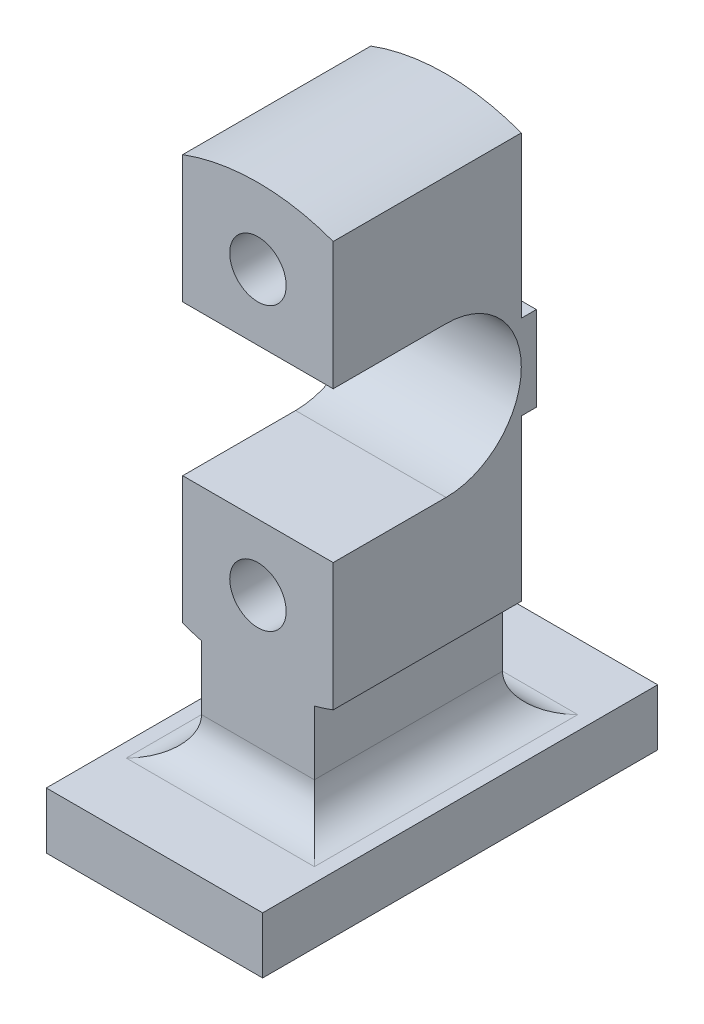
from build123d import *

# Parameters (mm, degrees)
UPRIGHT_PROFILE_SKETCH_R    = 15
UPRIGHT_BODY_DEPTH          = 50
BASE_PLATE_SKETCH_W         = 115
BASE_PLATE_SKETCH_H         = 210
BASE_PLATE_210X115X30_DEPTH = 30
BASE_BLEND_FILLET_R20_R     = 20
SIDE_BOSS_SKETCH_W          = 8
SIDE_BOSS_SKETCH_H          = 45
SIDE_BOSS_DEPTH             = 80
UPRIGHT_PROFILE_CUT_DEPTH   = 80


with BuildPart() as part:
    # Upright Profile Sketch → Upright Body (new, symmetric)
    with BuildSketch(Plane.XY):
        with BuildLine():
            Line((-40, -107.819293264), (-40, 107.819293264))
            ThreePointArc((-40, 107.819293264), (0, 115), (40, 107.819293264))
            Line((40, 107.819293264), (40, -107.819293264))
            ThreePointArc((40, -107.819293264), (35.036523196, -109.532835453), (30, -111.018016556))
            Line((30, -111.018016556), (30, -165))
            Line((30, -165), (-30, -165))
            Line((-30, -165), (-30, -111.018016556))
            ThreePointArc((-30, -111.018016556), (-35.036523196, -109.532835453), (-40, -107.819293264))
        make_face()
        with Locations((0, 75)):
            Circle(UPRIGHT_PROFILE_SKETCH_R, mode=Mode.SUBTRACT)
        with Locations(Location((0, -75, 0), (0, 0, 180))):
            Circle(UPRIGHT_PROFILE_SKETCH_R, mode=Mode.SUBTRACT)
    extrude(amount=UPRIGHT_BODY_DEPTH, both=True)

    # Base Plate Sketch → Base Plate 210x115x30 (add)
    with BuildSketch(Plane.XZ.offset(165)):
        Rectangle(BASE_PLATE_SKETCH_W, BASE_PLATE_SKETCH_H)
    extrude(amount=BASE_PLATE_210X115X30_DEPTH)

    # Base Blend Fillet R20
    base_blend_fillet_r20_edges = [part.edges().sort_by_distance(p)[0] for p in [
        (30, -165, 0),
        (-30, -165, 0),
        (0, -165, 50),
        (0, -165, -50),
    ]]
    fillet(base_blend_fillet_r20_edges, radius=BASE_BLEND_FILLET_R20_R)

    # Side Boss Sketch → Side Boss (add)
    with BuildSketch(Plane(origin=(40, 0, 0), x_dir=(0, 0, -1), z_dir=(1, 0, 0))):
        with Locations((54, 0)):
            Rectangle(SIDE_BOSS_SKETCH_W, SIDE_BOSS_SKETCH_H)
    extrude(amount=-SIDE_BOSS_DEPTH)

    # Upright Cut Sketch → Upright Profile Cut (cut)
    with BuildSketch(Plane(origin=(40, 0, 0), x_dir=(0, 0, -1), z_dir=(1, 0, 0))):
        with BuildLine():
            Line((10, 40), (-50, 40))
            Line((-50, 40), (-50, -40))
            Line((-50, -40), (10, -40))
            ThreePointArc((10, -40), (50, 0), (10, 40))
        make_face()
    extrude(amount=-UPRIGHT_PROFILE_CUT_DEPTH, mode=Mode.SUBTRACT)


solid = part.part
